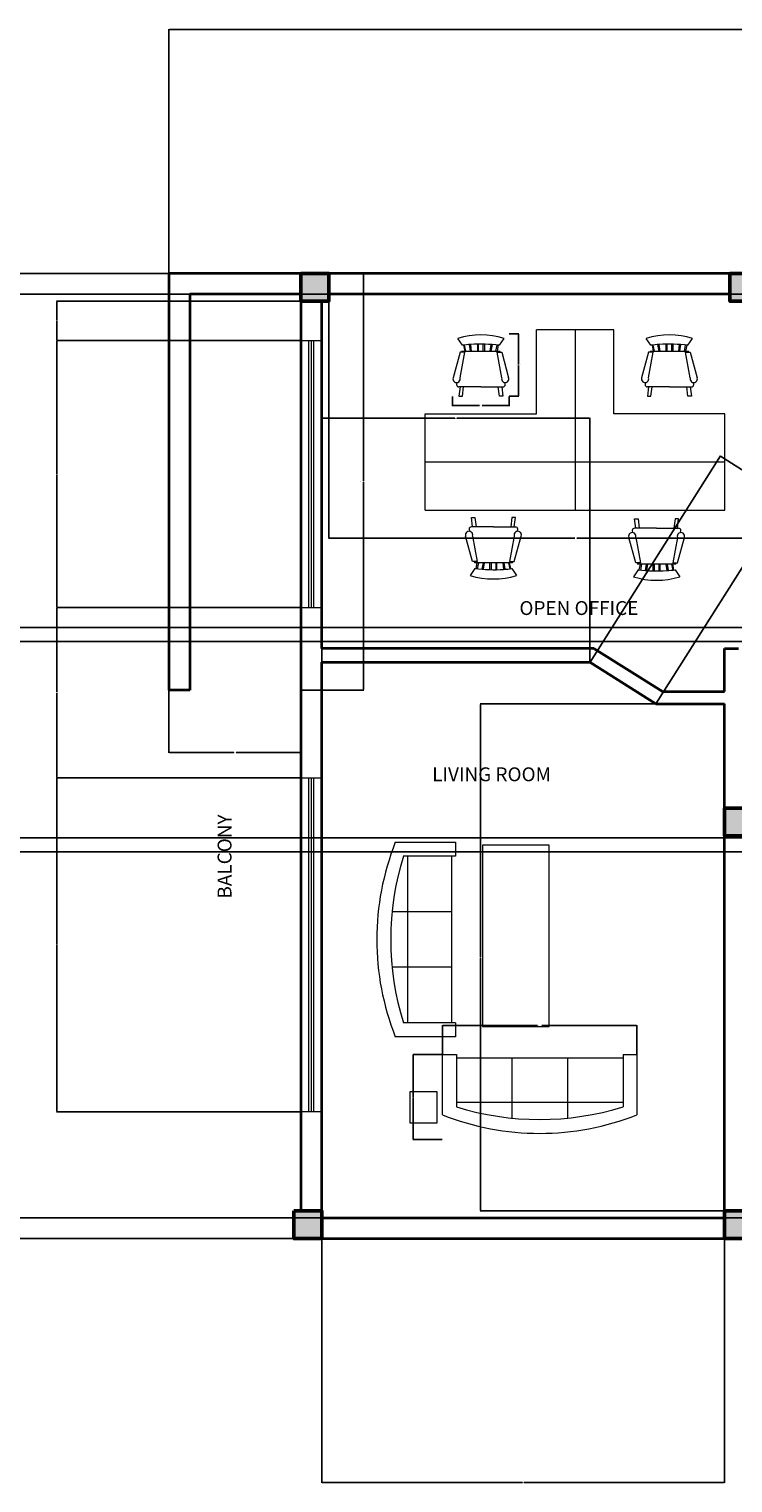
# Model space of a CAD drawing. Units: inches. Extents: x 369 to 4994, y 516 to 1297.
# Tile 4 of 9: x 1148 to 1452, y 516 to 1144. Entities that reach past the tile are written whole.
import ezdxf

# ---------------------------------------------------------------- set-up
doc = ezdxf.new("R2010")
doc.units = ezdxf.units.IN
doc.header["$MEASUREMENT"] = 0
for name, color, linetype, lineweight in [('A-ANNO-DIMS', 2, 'Continuous', 18), ('A-AREA-IDEN', 7, 'Continuous', 18), ('A-COLS', 7, 'Continuous', 50), ('A-FURN', 8, 'Continuous', 18), ('A-GLAZ', 4, 'Continuous', 18), ('A-WALL', 7, 'Continuous', 35)]:
    doc.layers.add(name, color=color, linetype=linetype, lineweight=lineweight)
doc.layers.add('A-COLS-PATT', color=18, linetype='Continuous', lineweight=13, true_color=0x000000)
doc.styles.get("Standard").update_dxf_attribs({"font": 'arial.ttf'})
doc.dimstyles.get("Standard").update_dxf_attribs({"dimtxt": 0.18, "dimasz": 0.18, "dimexe": 0.18, "dimexo": 0.0625, "dimgap": 0.09, "dimtad": 0, "dimtih": 1, "dimtoh": 1, "dimdec": 4, "dimzin": 0, "dimdsep": 46, "dimtxsty": 'Standard', "dimcen": 0.09, "dimadec": 0, "dimazin": 0, "dimtfac": 1, "dimtdec": 4, "dimtofl": 0, "dimtmove": 0, "dimatfit": 3, "dimfxl": 1, "dimtolj": 1, "dimtzin": 0, "dimarcsym": 0})

# ---------------------------------------------------------------- blocks, each defined once
blk = doc.blocks.new('Chair - Rocking')
for p, q in [((-8, -4.5), (-10, -1.5)), ((-7.5, -4.5), (-7, -7)), ((-6.5, -7), (-7.02225, -4.43)), ((-4.5, -7), (-4.96674, -4.19951)), ((-4, -7), (-4.40532, -4.16272)), ((-1.5, -4.05012), (-1.5, -7)), ((-1, -7), (-1, -4.05012)), ((1, -7), (1, -4.04655)), ((1.5, -4.05012), (1.5, -7)), ((4, -7), (4.40187, -4.18694)), ((4.5, -7), (4.96761, -4.19437)), ((6.5, -7), (7, -4.4057)), ((7.5, -4.5), (7, -7)), ((8, -4.5), (10, -1.5)), ((-9, -7.5), (-12, -18.49999)), ((-7, -7.5), (-9, -7.5)), ((-9, -18.49999), (-7, -7.5)), ((-8.23428, -6.99939), (-8.3093, -7.47958)), ((-8.23041, -7), (8.23915, -7)), ((7, -7.5), (9, -7.5)), ((9, -18.49999), (7, -7.5)), ((8.31071, -7.48854), (8.23449, -7.00073)), ((9, -7.5), (12, -18.49999)), ((-10.36644, -20.64523), (-10.5, -21.49999)), ((-9, -22.49999), (-9.5, -26.49999)), ((0, -22.49999), (-9.5, -22.49999)), ((-8, -26.49999), (-7.5, -22.49999)), ((0, -22.49999), (9.5, -22.49999)), ((8, -26.49999), (7.5, -22.49999)), ((9, -22.49999), (9.5, -26.49999)), ((10.5, -21.49999), (10.3575, -20.58798)), ((-9.5, -26.49999), (-8, -26.49999)), ((9.5, -26.49999), (8, -26.49999))]:
    blk.add_line(p, q)
for centre, radius, start, end in [((0, -34.08333), 34.08333, 72.93847, 107.0615), ((0, -68.25004), 64.25, 93.92211, 97.15267), ((0, -68.25004), 64.25, 82.84733, 93.92211), ((-10.5, -18.99999), 1.58114, 161.5651, 18.43495), ((10.5, -18.99999), 1.58114, 161.5651, 18.43495), ((-9.5, -21.49999), 1, 180, 270), ((9.5, -21.49999), 1, 270, 0)]:
    blk.add_arc(centre, radius, start, end)
blk = doc.blocks.new('Sofa - Roundback 7 ft.')
for p, q in [((-36.000027, -34), (-36.000027, -11.4696)), ((-12.00002, -32.4421), (-12.00003, -6.5971)), ((11.99997, -32.4421), (11.99998, -6.5971)), ((35.99998, -34), (35.99998, -11.4696)), ((-35.999844, -13.3819), (35.9998, -13.3819)), ((-36.000027, -32.4421), (35.99998, -32.4421))]:
    blk.add_line(p, q)
for points in [[(-36.000027, -34), (-42.000027, -34), (-42.000027, -8)], [(41.99998, -8), (41.99998, -34), (35.99998, -34)]]:
    blk.add_lwpolyline(points)
for centre, radius, start, end in [((0, -114.25), 114.25, 68.43141, 111.5686), ((-0.00001, -127.1968), 121.1968, 72.72033, 107.2797)]:
    blk.add_arc(centre, radius, start, end)
blk = doc.blocks.new('BALCONY-EDGE')
for p, q in [((57, 180), (0, 180)), ((0, 180), (0, 0)), ((9, 171), (9, 0)), ((57, 171), (9, 171)), ((9, 0), (0, 0))]:
    blk.add_line(p, q)
blk = doc.blocks.new('*D13')
at = {"layer": 'A-ANNO-DIMS', "color": 0, "lineweight": -2, "transparency": 16777216}
for p, q in [((1265.44, 1038.79), (1292.55, 1038.79)), ((1292.37, 1038.61), (1292.37, 948.97)), ((1292.37, 858.97), (1292.37, 948.61)), ((1265.44, 858.79), (1292.55, 858.79))]:
    blk.add_line(p, q, dxfattribs=at)
at = {"layer": 'A-ANNO-DIMS', "color": 0, "transparency": 16777216}
for points in [[(1292.34, 1038.61), (1292.4, 1038.61), (1292.37, 1038.79)], [(1292.34, 858.97), (1292.4, 858.97), (1292.37, 858.79)]]:
    blk.add_solid(points, dxfattribs=at)
at = {"layer": 'Defpoints', "color": 0, "transparency": 16777216}
for p in [(1265.37, 1038.79), (1292.37, 1038.79), (1265.37, 858.79)]:
    blk.add_point(p, dxfattribs=at)
at = {"layer": 'A-ANNO-DIMS', "color": 0, "transparency": 16777216, "insert": (1292.37, 948.79), "char_height": 0.18, "attachment_point": 5}
blk.add_mtext('\\A1;BALCONY EDGE 180 TYP.', dxfattribs=at)
blk = doc.blocks.new('*D14')
at = {"layer": 'A-ANNO-DIMS', "color": 0, "lineweight": -2, "transparency": 16777216}
for p, q in [((1208.37, 858.73), (1208.37, 831.61)), ((1265.37, 858.73), (1265.37, 831.61)), ((1208.55, 831.79), (1236.35, 831.79)), ((1265.19, 831.79), (1237.4, 831.79))]:
    blk.add_line(p, q, dxfattribs=at)
at = {"layer": 'A-ANNO-DIMS', "color": 0, "transparency": 16777216}
for points in [[(1208.55, 831.82), (1208.55, 831.76), (1208.37, 831.79)], [(1265.19, 831.82), (1265.19, 831.76), (1265.37, 831.79)]]:
    blk.add_solid(points, dxfattribs=at)
at = {"layer": 'Defpoints', "color": 0, "transparency": 16777216}
for p in [(1208.37, 858.79), (1265.37, 858.79), (1265.37, 831.79)]:
    blk.add_point(p, dxfattribs=at)
at = {"layer": 'A-ANNO-DIMS', "color": 0, "transparency": 16777216, "insert": (1236.87, 831.79), "char_height": 0.18, "attachment_point": 5}
blk.add_mtext('\\A1;57 TYP.', dxfattribs=at)
blk = doc.blocks.new('*D21')
at = {"layer": 'A-ANNO-DIMS', "color": 0, "lineweight": -2, "transparency": 16777216}
for p, q in [((1326.51, 701.31), (1326.51, 714.03)), ((1326.69, 713.85), (1367.6, 713.85)), ((1410.33, 713.85), (1369.41, 713.85)), ((1410.51, 701.31), (1410.51, 714.03))]:
    blk.add_line(p, q, dxfattribs=at)
at = {"layer": 'A-ANNO-DIMS', "color": 0, "transparency": 16777216}
for points in [[(1326.69, 713.88), (1326.69, 713.82), (1326.51, 713.85)], [(1410.33, 713.88), (1410.33, 713.82), (1410.51, 713.85)]]:
    blk.add_solid(points, dxfattribs=at)
at = {"layer": 'Defpoints', "color": 0, "transparency": 16777216}
for p in [(1326.51, 713.85), (1326.51, 701.25), (1410.51, 701.25)]:
    blk.add_point(p, dxfattribs=at)
at = {"layer": 'A-ANNO-DIMS', "color": 0, "transparency": 16777216, "insert": (1368.51, 713.85), "char_height": 0.18, "attachment_point": 5}
blk.add_mtext('\\A1;SOFA 84 TYP.', dxfattribs=at)
blk = doc.blocks.new('*D22')
at = {"layer": 'A-ANNO-DIMS', "color": 0, "lineweight": -2, "transparency": 16777216}
for p, q in [((1326.44, 701.25), (1313.73, 701.25)), ((1313.91, 701.07), (1313.91, 683.09)), ((1313.91, 664.76), (1313.91, 682.73)), ((1326.44, 664.58), (1313.73, 664.58))]:
    blk.add_line(p, q, dxfattribs=at)
at = {"layer": 'A-ANNO-DIMS', "color": 0, "transparency": 16777216}
for points in [[(1313.88, 701.07), (1313.94, 701.07), (1313.91, 701.25)], [(1313.88, 664.76), (1313.94, 664.76), (1313.91, 664.58)]]:
    blk.add_solid(points, dxfattribs=at)
at = {"layer": 'Defpoints', "color": 0, "transparency": 16777216}
for p in [(1326.51, 701.25), (1313.91, 664.58), (1326.51, 664.58)]:
    blk.add_point(p, dxfattribs=at)
at = {"layer": 'A-ANNO-DIMS', "color": 0, "transparency": 16777216, "insert": (1313.91, 682.91), "char_height": 0.18, "attachment_point": 5}
blk.add_mtext('\\A1;37 TYP.', dxfattribs=at)
blk = doc.blocks.new('*D23')
at = {"layer": 'A-ANNO-DIMS', "color": 0, "lineweight": -2, "transparency": 16777216}
for p, q in [((1355.39, 1012.74), (1359.55, 1012.74)), ((1359.37, 1012.56), (1359.37, 999.42)), ((1359.37, 985.92), (1359.37, 999.06)), ((1355.39, 985.74), (1359.55, 985.74))]:
    blk.add_line(p, q, dxfattribs=at)
at = {"layer": 'A-ANNO-DIMS', "color": 0, "transparency": 16777216}
for points in [[(1359.34, 1012.56), (1359.4, 1012.56), (1359.37, 1012.74)], [(1359.34, 985.92), (1359.4, 985.92), (1359.37, 985.74)]]:
    blk.add_solid(points, dxfattribs=at)
at = {"layer": 'Defpoints', "color": 0, "transparency": 16777216}
for p in [(1355.32, 1012.74), (1359.37, 1012.74), (1355.32, 985.74)]:
    blk.add_point(p, dxfattribs=at)
at = {"layer": 'A-ANNO-DIMS', "color": 0, "transparency": 16777216, "insert": (1359.37, 999.24), "char_height": 0.18, "attachment_point": 5}
blk.add_mtext('\\A1;CHAIR 27 TYP.', dxfattribs=at)
blk = doc.blocks.new('*D24')
at = {"layer": 'A-ANNO-DIMS', "color": 0, "lineweight": -2, "transparency": 16777216}
for p, q in [((1330.89, 985.68), (1330.89, 981.51)), ((1331.07, 981.69), (1342.58, 981.69)), ((1355.14, 981.69), (1343.64, 981.69)), ((1355.32, 985.68), (1355.32, 981.51))]:
    blk.add_line(p, q, dxfattribs=at)
at = {"layer": 'A-ANNO-DIMS', "color": 0, "transparency": 16777216}
for points in [[(1331.07, 981.72), (1331.07, 981.66), (1330.89, 981.69)], [(1355.14, 981.72), (1355.14, 981.66), (1355.32, 981.69)]]:
    blk.add_solid(points, dxfattribs=at)
at = {"layer": 'Defpoints', "color": 0, "transparency": 16777216}
for p in [(1330.89, 985.74), (1355.32, 985.74), (1355.32, 981.69)]:
    blk.add_point(p, dxfattribs=at)
at = {"layer": 'A-ANNO-DIMS', "color": 0, "transparency": 16777216, "insert": (1343.11, 981.69), "char_height": 0.18, "attachment_point": 5}
blk.add_mtext('\\A1;24 TYP.', dxfattribs=at)
blk = doc.blocks.new('*D46')
at = {"layer": 'A-ANNO-DIMS', "color": 0, "lineweight": -2, "transparency": 16777216}
for p, q in [((978.32, 1029.79), (2671.51, 1029.79)), ((2671.33, 1029.61), (2671.33, 957.97)), ((2671.33, 885.97), (2671.33, 957.61)), ((1038.32, 885.79), (2671.51, 885.79))]:
    blk.add_line(p, q, dxfattribs=at)
at = {"layer": 'A-ANNO-DIMS', "color": 0, "transparency": 16777216}
for points in [[(2671.3, 1029.61), (2671.36, 1029.61), (2671.33, 1029.79)], [(2671.3, 885.97), (2671.36, 885.97), (2671.33, 885.79)]]:
    blk.add_solid(points, dxfattribs=at)
at = {"layer": 'Defpoints', "color": 0, "transparency": 16777216}
for p in [(978.26, 1029.79), (2671.33, 1029.79), (1038.26, 885.79)]:
    blk.add_point(p, dxfattribs=at)
at = {"layer": 'A-ANNO-DIMS', "color": 0, "transparency": 16777216, "insert": (2671.33, 957.79), "char_height": 0.18, "attachment_point": 5}
blk.add_mtext('\\A1;144', dxfattribs=at)
blk = doc.blocks.new('*D47')
at = {"layer": 'A-ANNO-DIMS', "color": 0, "lineweight": -2, "transparency": 16777216}
for p, q in [((1038.32, 879.79), (2671.51, 879.79)), ((2671.33, 879.61), (2671.33, 837.52)), ((2671.33, 795.07), (2671.33, 837.16)), ((1035.32, 794.89), (2671.51, 794.89))]:
    blk.add_line(p, q, dxfattribs=at)
at = {"layer": 'A-ANNO-DIMS', "color": 0, "transparency": 16777216}
for points in [[(2671.3, 879.61), (2671.36, 879.61), (2671.33, 879.79)], [(2671.3, 795.07), (2671.36, 795.07), (2671.33, 794.89)]]:
    blk.add_solid(points, dxfattribs=at)
at = {"layer": 'Defpoints', "color": 0, "transparency": 16777216}
for p in [(1038.26, 879.79), (2671.33, 879.79), (1035.26, 794.89)]:
    blk.add_point(p, dxfattribs=at)
at = {"layer": 'A-ANNO-DIMS', "color": 0, "transparency": 16777216, "insert": (2671.33, 837.34), "char_height": 0.18, "attachment_point": 5}
blk.add_mtext('\\A1;84.9', dxfattribs=at)
blk = doc.blocks.new('*D52')
at = {"layer": 'A-ANNO-DIMS', "color": 0, "lineweight": -2, "transparency": 16777216}
for p, q in [((942.32, 788.89), (2671.51, 788.89)), ((2671.33, 788.71), (2671.33, 710.02)), ((2671.33, 630.97), (2671.33, 709.66)), ((1035.32, 630.79), (2671.51, 630.79))]:
    blk.add_line(p, q, dxfattribs=at)
at = {"layer": 'A-ANNO-DIMS', "color": 0, "transparency": 16777216}
for points in [[(2671.3, 788.71), (2671.36, 788.71), (2671.33, 788.89)], [(2671.3, 630.97), (2671.36, 630.97), (2671.33, 630.79)]]:
    blk.add_solid(points, dxfattribs=at)
at = {"layer": 'Defpoints', "color": 0, "transparency": 16777216}
for p in [(942.26, 788.89), (2671.33, 788.89), (1035.26, 630.79)]:
    blk.add_point(p, dxfattribs=at)
at = {"layer": 'A-ANNO-DIMS', "color": 0, "transparency": 16777216, "insert": (2671.33, 709.84), "char_height": 0.18, "attachment_point": 5}
blk.add_mtext('\\A1;158.1', dxfattribs=at)
blk = doc.blocks.new('*D74')
at = {"layer": 'A-ANNO-DIMS', "color": 0, "lineweight": -2, "transparency": 16777216}
for p, q in [((1208.37, 1038.85), (1208.37, 1144.37)), ((1208.55, 1144.19), (1494.58, 1144.19)), ((1781.19, 1144.19), (1495.16, 1144.19)), ((1781.37, 1038.85), (1781.37, 1144.37))]:
    blk.add_line(p, q, dxfattribs=at)
at = {"layer": 'A-ANNO-DIMS', "color": 0, "transparency": 16777216}
for points in [[(1208.55, 1144.22), (1208.55, 1144.16), (1208.37, 1144.19)], [(1781.19, 1144.22), (1781.19, 1144.16), (1781.37, 1144.19)]]:
    blk.add_solid(points, dxfattribs=at)
at = {"layer": 'Defpoints', "color": 0, "transparency": 16777216}
for p in [(1781.37, 1144.19), (1208.37, 1038.79), (1781.37, 1038.79)]:
    blk.add_point(p, dxfattribs=at)
at = {"layer": 'A-ANNO-DIMS', "color": 0, "transparency": 16777216, "insert": (1494.87, 1144.19), "char_height": 0.18, "attachment_point": 5}
blk.add_mtext('\\A1;573', dxfattribs=at)
blk = doc.blocks.new('*D75')
at = {"layer": 'A-ANNO-DIMS', "color": 0, "lineweight": -2, "transparency": 16777216}
for p, q in [((1208.31, 1038.79), (368.68, 1038.79)), ((368.86, 1038.61), (368.86, 830.47)), ((368.86, 621.97), (368.86, 830.11)), ((1262.31, 621.79), (368.68, 621.79))]:
    blk.add_line(p, q, dxfattribs=at)
at = {"layer": 'A-ANNO-DIMS', "color": 0, "transparency": 16777216}
for points in [[(368.83, 1038.61), (368.89, 1038.61), (368.86, 1038.79)], [(368.83, 621.97), (368.89, 621.97), (368.86, 621.79)]]:
    blk.add_solid(points, dxfattribs=at)
at = {"layer": 'Defpoints', "color": 0, "transparency": 16777216}
for p in [(368.86, 1038.79), (1208.37, 1038.79), (1262.37, 621.79)]:
    blk.add_point(p, dxfattribs=at)
at = {"layer": 'A-ANNO-DIMS', "color": 0, "transparency": 16777216, "insert": (368.86, 830.29), "char_height": 0.18, "attachment_point": 5}
blk.add_mtext('\\A1;417', dxfattribs=at)
blk = doc.blocks.new('*D76')
at = {"layer": 'A-ANNO-DIMS', "color": 0, "lineweight": -2, "transparency": 16777216}
for p, q in [((1277.37, 1029.73), (1277.37, 924.21)), ((1490.89, 1029.73), (1490.89, 924.21)), ((1277.55, 924.39), (1383.74, 924.39)), ((1490.71, 924.39), (1384.53, 924.39))]:
    blk.add_line(p, q, dxfattribs=at)
at = {"layer": 'A-ANNO-DIMS', "color": 0, "transparency": 16777216}
for points in [[(1277.55, 924.42), (1277.55, 924.36), (1277.37, 924.39)], [(1490.71, 924.42), (1490.71, 924.36), (1490.89, 924.39)]]:
    blk.add_solid(points, dxfattribs=at)
at = {"layer": 'Defpoints', "color": 0, "transparency": 16777216}
for p in [(1277.37, 1029.79), (1490.89, 1029.79), (1277.37, 924.39)]:
    blk.add_point(p, dxfattribs=at)
at = {"layer": 'A-ANNO-DIMS', "color": 0, "transparency": 16777216, "insert": (1384.13, 924.39), "char_height": 0.18, "attachment_point": 5}
blk.add_mtext('\\A1;213.5', dxfattribs=at)
blk = doc.blocks.new('*D81')
at = {"layer": 'A-ANNO-DIMS', "color": 0, "lineweight": -2, "transparency": 16777216}
for p, q in [((1274.37, 630.73), (1274.37, 516.21)), ((1448.37, 630.73), (1448.37, 516.21)), ((1274.55, 516.39), (1361.09, 516.39)), ((1448.19, 516.39), (1361.65, 516.39))]:
    blk.add_line(p, q, dxfattribs=at)
at = {"layer": 'A-ANNO-DIMS', "color": 0, "transparency": 16777216}
for points in [[(1274.55, 516.42), (1274.55, 516.36), (1274.37, 516.39)], [(1448.19, 516.42), (1448.19, 516.36), (1448.37, 516.39)]]:
    blk.add_solid(points, dxfattribs=at)
at = {"layer": 'Defpoints', "color": 0, "transparency": 16777216}
for p in [(1274.37, 630.79), (1448.37, 630.79), (1448.37, 516.39)]:
    blk.add_point(p, dxfattribs=at)
at = {"layer": 'A-ANNO-DIMS', "color": 0, "transparency": 16777216, "insert": (1361.37, 516.39), "char_height": 0.18, "attachment_point": 5}
blk.add_mtext('\\A1;174', dxfattribs=at)
blk = doc.blocks.new('*D87')
at = {"layer": 'A-ANNO-DIMS', "color": 0, "lineweight": -2, "transparency": 16777216}
for p, q in [((1274.37, 870.85), (1274.37, 976.37)), ((1274.55, 976.19), (1331.85, 976.19)), ((1390.05, 976.19), (1332.76, 976.19)), ((1390.23, 870.85), (1390.23, 976.37))]:
    blk.add_line(p, q, dxfattribs=at)
at = {"layer": 'A-ANNO-DIMS', "color": 0, "transparency": 16777216}
for points in [[(1274.55, 976.22), (1274.55, 976.16), (1274.37, 976.19)], [(1390.05, 976.22), (1390.05, 976.16), (1390.23, 976.19)]]:
    blk.add_solid(points, dxfattribs=at)
at = {"layer": 'Defpoints', "color": 0, "transparency": 16777216}
for p in [(1390.23, 976.19), (1274.37, 870.79), (1390.23, 870.79)]:
    blk.add_point(p, dxfattribs=at)
at = {"layer": 'A-ANNO-DIMS', "color": 0, "transparency": 16777216, "insert": (1332.3, 976.19), "char_height": 0.18, "attachment_point": 5}
blk.add_mtext('\\A1;115.86', dxfattribs=at)
blk = doc.blocks.new('*D88')
at = {"layer": 'A-ANNO-DIMS', "color": 0, "lineweight": -2, "transparency": 16777216}
for p, q in [((1390.27, 870.84), (1446.63, 960.04)), ((1446.68, 959.8), (1460.49, 951.07)), ((1474.87, 941.99), (1461.06, 950.71)), ((1418.75, 852.84), (1475.12, 942.04))]:
    blk.add_line(p, q, dxfattribs=at)
at = {"layer": 'A-ANNO-DIMS', "color": 0, "transparency": 16777216}
for points in [[(1446.7, 959.82), (1446.67, 959.77), (1446.53, 959.89)], [(1474.88, 942.01), (1474.85, 941.96), (1475.02, 941.89)]]:
    blk.add_solid(points, dxfattribs=at)
at = {"layer": 'Defpoints', "color": 0, "transparency": 16777216}
for p in [(1475.02, 941.89), (1390.23, 870.79), (1418.72, 852.79)]:
    blk.add_point(p, dxfattribs=at)
at = {"layer": 'A-ANNO-DIMS', "color": 0, "transparency": 16777216, "insert": (1460.78, 950.89), "char_height": 0.18, "attachment_point": 5}
blk.add_mtext('\\A1;33.7', dxfattribs=at)
blk = doc.blocks.new('*D89')
at = {"layer": 'A-ANNO-DIMS', "color": 0, "lineweight": -2, "transparency": 16777216}
for p, q in [((1448.31, 852.79), (1342.79, 852.79)), ((1342.97, 852.61), (1342.97, 743.47)), ((1342.97, 633.97), (1342.97, 743.11)), ((1448.31, 633.79), (1342.79, 633.79))]:
    blk.add_line(p, q, dxfattribs=at)
at = {"layer": 'A-ANNO-DIMS', "color": 0, "transparency": 16777216}
for points in [[(1342.94, 852.61), (1343, 852.61), (1342.97, 852.79)], [(1342.94, 633.97), (1343, 633.97), (1342.97, 633.79)]]:
    blk.add_solid(points, dxfattribs=at)
at = {"layer": 'Defpoints', "color": 0, "transparency": 16777216}
for p in [(1342.97, 852.79), (1448.37, 852.79), (1448.37, 633.79)]:
    blk.add_point(p, dxfattribs=at)
at = {"layer": 'A-ANNO-DIMS', "color": 0, "transparency": 16777216, "insert": (1342.97, 743.29), "char_height": 0.18, "attachment_point": 5}
blk.add_mtext('\\A1;219', dxfattribs=at)
blk = doc.blocks.new('*D90')
at = {"layer": 'A-ANNO-DIMS', "color": 0, "lineweight": -2, "transparency": 16777216}
for p, q in [((1265.31, 1026.79), (1159.79, 1026.79)), ((1159.97, 1026.61), (1159.97, 1018.46)), ((1159.97, 1009.95), (1159.97, 1018.1)), ((1265.31, 1009.77), (1159.79, 1009.77))]:
    blk.add_line(p, q, dxfattribs=at)
at = {"layer": 'A-ANNO-DIMS', "color": 0, "transparency": 16777216}
for points in [[(1159.94, 1026.61), (1160, 1026.61), (1159.97, 1026.79)], [(1159.94, 1009.95), (1160, 1009.95), (1159.97, 1009.77)]]:
    blk.add_solid(points, dxfattribs=at)
at = {"layer": 'Defpoints', "color": 0, "transparency": 16777216}
for p in [(1159.97, 1026.79), (1265.37, 1026.79), (1265.37, 1009.77)]:
    blk.add_point(p, dxfattribs=at)
at = {"layer": 'A-ANNO-DIMS', "color": 0, "transparency": 16777216, "insert": (1159.97, 1018.28), "char_height": 0.18, "attachment_point": 5}
blk.add_mtext('\\A1;17.023', dxfattribs=at)
blk = doc.blocks.new('*D91')
at = {"layer": 'A-ANNO-DIMS', "color": 0, "lineweight": -2, "transparency": 16777216}
for p, q in [((1265.31, 1009.77), (1159.79, 1009.77)), ((1159.97, 1009.59), (1159.97, 952.25)), ((1159.97, 894.56), (1159.97, 951.89)), ((1265.31, 894.38), (1159.79, 894.38))]:
    blk.add_line(p, q, dxfattribs=at)
at = {"layer": 'A-ANNO-DIMS', "color": 0, "transparency": 16777216}
for points in [[(1159.94, 1009.59), (1160, 1009.59), (1159.97, 1009.77)], [(1159.94, 894.56), (1160, 894.56), (1159.97, 894.38)]]:
    blk.add_solid(points, dxfattribs=at)
at = {"layer": 'Defpoints', "color": 0, "transparency": 16777216}
for p in [(1159.97, 1009.77), (1265.37, 1009.77), (1265.37, 894.38)]:
    blk.add_point(p, dxfattribs=at)
at = {"layer": 'A-ANNO-DIMS', "color": 0, "transparency": 16777216, "insert": (1159.97, 952.07), "char_height": 0.18, "attachment_point": 5}
blk.add_mtext('\\A1;115.39', dxfattribs=at)
blk = doc.blocks.new('*D92')
at = {"layer": 'A-ANNO-DIMS', "color": 0, "lineweight": -2, "transparency": 16777216}
for p, q in [((1265.31, 894.38), (1159.79, 894.38)), ((1159.97, 894.2), (1159.97, 857.81)), ((1159.97, 821.05), (1159.97, 857.44)), ((1265.31, 820.87), (1159.79, 820.87))]:
    blk.add_line(p, q, dxfattribs=at)
at = {"layer": 'A-ANNO-DIMS', "color": 0, "transparency": 16777216}
for points in [[(1159.94, 894.2), (1160, 894.2), (1159.97, 894.38)], [(1159.94, 821.05), (1160, 821.05), (1159.97, 820.87)]]:
    blk.add_solid(points, dxfattribs=at)
at = {"layer": 'Defpoints', "color": 0, "transparency": 16777216}
for p in [(1159.97, 894.38), (1265.37, 894.38), (1265.37, 820.87)]:
    blk.add_point(p, dxfattribs=at)
at = {"layer": 'A-ANNO-DIMS', "color": 0, "transparency": 16777216, "insert": (1159.97, 857.62), "char_height": 0.18, "attachment_point": 5}
blk.add_mtext('\\A1;73.51', dxfattribs=at)
blk = doc.blocks.new('*D93')
at = {"layer": 'A-ANNO-DIMS', "color": 0, "lineweight": -2, "transparency": 16777216}
for p, q in [((1265.31, 820.87), (1159.79, 820.87)), ((1159.97, 820.69), (1159.97, 748.88)), ((1159.97, 676.7), (1159.97, 748.51)), ((1265.31, 676.52), (1159.79, 676.52))]:
    blk.add_line(p, q, dxfattribs=at)
at = {"layer": 'A-ANNO-DIMS', "color": 0, "transparency": 16777216}
for points in [[(1159.94, 820.69), (1160, 820.69), (1159.97, 820.87)], [(1159.94, 676.7), (1160, 676.7), (1159.97, 676.52)]]:
    blk.add_solid(points, dxfattribs=at)
at = {"layer": 'Defpoints', "color": 0, "transparency": 16777216}
for p in [(1159.97, 820.87), (1265.37, 820.87), (1265.37, 676.52)]:
    blk.add_point(p, dxfattribs=at)
at = {"layer": 'A-ANNO-DIMS', "color": 0, "transparency": 16777216, "insert": (1159.97, 748.69), "char_height": 0.18, "attachment_point": 5}
blk.add_mtext('\\A1;144.35', dxfattribs=at)
blk = doc.blocks.new('*D98')
at = {"layer": 'A-ANNO-DIMS', "color": 0, "lineweight": -2, "transparency": 16777216}
for p, q in [((1992.86, 1038.79), (368.68, 1038.79)), ((368.86, 1038.61), (368.86, 830.47)), ((368.86, 621.97), (368.86, 830.11)), ((2046.86, 621.79), (368.68, 621.79))]:
    blk.add_line(p, q, dxfattribs=at)
at = {"layer": 'A-ANNO-DIMS', "color": 0, "transparency": 16777216}
for points in [[(368.83, 1038.61), (368.89, 1038.61), (368.86, 1038.79)], [(368.83, 621.97), (368.89, 621.97), (368.86, 621.79)]]:
    blk.add_solid(points, dxfattribs=at)
at = {"layer": 'Defpoints', "color": 0, "transparency": 16777216}
for p in [(368.86, 1038.79), (1992.93, 1038.79), (2046.93, 621.79)]:
    blk.add_point(p, dxfattribs=at)
at = {"layer": 'A-ANNO-DIMS', "color": 0, "transparency": 16777216, "insert": (368.86, 830.29), "char_height": 0.18, "attachment_point": 5}
blk.add_mtext('\\A1;417', dxfattribs=at)

msp = doc.modelspace()

# ---------------------------------------------------------------- hatches: boundary and pattern name
at = {"layer": 'A-COLS-PATT'}
h = msp.add_hatch(color=256, dxfattribs=at)
h.dxf.hatch_style = 1
h.paths.add_polyline_path([(540.2581, 633.7894), (528.2581, 633.7894), (528.2581, 621.7894), (540.2581, 621.7894)])
h.paths.add_polyline_path([(726.2581, 633.7894), (714.2581, 633.7894), (714.2581, 621.7894), (726.2581, 621.7894)])
h.paths.add_polyline_path([(918.2581, 633.7894), (906.2581, 633.7894), (906.2581, 621.7894), (918.2581, 621.7894)])
h.paths.add_polyline_path([(1047.2581, 633.7894), (1035.2581, 633.7894), (1035.2581, 621.7894), (1047.2581, 621.7894)])
h.paths.add_polyline_path([(1047.2581, 798.6977), (1035.2581, 798.6977), (1035.2581, 786.6977), (1047.2581, 786.6977)])
h.paths.add_polyline_path([(918.2581, 795.7894), (906.2581, 795.7894), (906.2581, 783.7894), (918.2581, 783.7894)])
h.paths.add_polyline_path([(726.2581, 795.7894), (714.2581, 795.7894), (714.2581, 783.7894), (726.2581, 783.7894)])
h.paths.add_polyline_path([(1047.2581, 1038.7894), (1035.2581, 1038.7894), (1035.2581, 1026.7894), (1047.2581, 1026.7894)])
h.paths.add_polyline_path([(855.044, 1038.7894), (843.044, 1038.7894), (843.044, 1026.7894), (855.044, 1026.7894)])
h.paths.add_polyline_path([(728.5536, 1038.7894), (716.5536, 1038.7894), (716.5536, 1026.7894), (728.5536, 1026.7894)])
h.paths.add_polyline_path([(543.2581, 1038.7894), (531.2581, 1038.7894), (531.2581, 1026.7894), (543.2581, 1026.7894)])
h.paths.add_polyline_path([(543.2581, 792.9013), (531.2581, 792.9013), (531.2581, 780.9013), (543.2581, 780.9013), (543.2581, 783.7894)])
h.paths.add_polyline_path([(1274.3738, 633.7894), (1262.3738, 633.7894), (1262.3738, 621.7894), (1274.3738, 621.7894)])
h.paths.add_polyline_path([(1460.3738, 633.7894), (1448.3738, 633.7894), (1448.3738, 621.7894), (1460.3738, 621.7894)])
h.paths.add_polyline_path([(1652.3738, 633.7894), (1640.3738, 633.7894), (1640.3738, 621.7894), (1652.3738, 621.7894)])
h.paths.add_polyline_path([(1781.3738, 633.7894), (1769.3738, 633.7894), (1769.3738, 621.7894), (1781.3738, 621.7894)])
h.paths.add_polyline_path([(1781.3738, 1038.7894), (1769.3738, 1038.7894), (1769.3738, 1026.7894), (1781.3738, 1026.7894)])
h.paths.add_polyline_path([(1625.484, 1038.7894), (1613.484, 1038.7894), (1613.484, 1026.7894), (1615.6962, 1026.7894), (1625.484, 1026.7894)])
h.paths.add_polyline_path([(1462.6692, 1038.7894), (1450.6692, 1038.7894), (1450.6692, 1026.7894), (1462.6692, 1026.7894)])
h.paths.add_polyline_path([(1277.3738, 1038.7894), (1265.3738, 1038.7894), (1265.3738, 1026.7894), (1277.3738, 1026.7894)])
h.paths.add_polyline_path([(1460.3738, 807.7894), (1448.3738, 807.7894), (1448.3738, 795.7894), (1460.3738, 795.7894)])
h.paths.add_polyline_path([(1652.3738, 807.7894), (1640.3738, 807.7894), (1640.3738, 795.7894), (1652.3738, 795.7894)])
h.paths.add_polyline_path([(2244.9265, 633.7894), (2232.9265, 633.7894), (2232.9265, 621.7894), (2244.9265, 621.7894)])
h.paths.add_polyline_path([(2058.9265, 633.7894), (2046.9265, 633.7894), (2046.9265, 621.7894), (2058.9265, 621.7894)])
h.paths.add_polyline_path([(2436.9265, 633.7894), (2424.9265, 633.7894), (2424.9265, 621.7894), (2436.9265, 621.7894)])
h.paths.add_polyline_path([(2565.9265, 633.7894), (2553.9265, 633.7894), (2553.9265, 621.7894), (2565.9265, 621.7894)])
h.paths.add_polyline_path([(2565.9265, 798.6977), (2553.9265, 798.6977), (2553.9265, 786.6977), (2565.9265, 786.6977)])
h.paths.add_polyline_path([(2565.9265, 1038.7894), (2553.9265, 1038.7894), (2553.9265, 1026.7894), (2565.9265, 1026.7894)])
h.paths.add_polyline_path([(2436.9265, 1038.7894), (2424.9265, 1038.7894), (2424.9265, 1026.7894), (2436.9265, 1026.7894)])
h.paths.add_polyline_path([(2247.222, 1038.7894), (2235.222, 1038.7894), (2235.222, 1026.7894), (2247.222, 1026.7894)])
h.paths.add_polyline_path([(2061.9265, 1038.7894), (2049.9265, 1038.7894), (2049.9265, 1026.7894), (2061.9265, 1026.7894)])

# ---------------------------------------------------------------- linework, layer by layer
at = {"layer": 'A-COLS'}
for points in [[(1265.3738, 1038.7894), (1277.3738, 1038.7894), (1277.3738, 1026.7894), (1265.3738, 1026.7894)], [(1450.6692, 1038.7894), (1462.6692, 1038.7894), (1462.6692, 1026.7894), (1450.6692, 1026.7894)], [(1448.3738, 807.7894), (1460.3738, 807.7894), (1460.3738, 795.7894), (1448.3738, 795.7894)], [(1262.3738, 633.7894), (1274.3738, 633.7894), (1274.3738, 621.7894), (1262.3738, 621.7894)], [(1448.3738, 633.7894), (1460.3738, 633.7894), (1460.3738, 621.7894), (1448.3738, 621.7894)]]:
    msp.add_lwpolyline(points, close=True, dxfattribs=at)
at = {"layer": 'A-FURN'}
for p, q in [((1367.1047, 978.1573), (1367.1047, 1014.4875)), ((1400.5573, 1014.4875), (1367.1047, 1014.4875)), ((1383.831, 1014.4875), (1383.831, 936.4987)), ((1400.5573, 978.1573), (1400.5573, 1014.4875)), ((1319.1076, 936.4987), (1319.1076, 978.1573)), ((1319.1076, 978.1573), (1367.1047, 978.1573)), ((1448.5544, 978.1573), (1400.5573, 978.1573)), ((1448.5544, 936.4987), (1448.5544, 978.1573)), ((1319.1076, 957.328), (1448.5544, 957.328)), ((1319.1076, 936.4987), (1448.5544, 936.4987))]:
    msp.add_line(p, q, dxfattribs=at)
for points in [[(1343.7905, 713.4743), (1372.6633, 713.4743), (1372.6633, 791.7062), (1343.7905, 791.7062)], [(1312.4848, 671.8573), (1324.2157, 671.8573), (1324.2157, 685.1152), (1312.4848, 685.1152)]]:
    msp.add_lwpolyline(points, close=True, dxfattribs=at)
at = {"layer": 'A-GLAZ'}
for p, q in [((1268.7977, 894.3793), (1268.7977, 1009.766)), ((1269.8738, 894.3793), (1269.8738, 1009.766)), ((1270.9499, 894.3793), (1270.9499, 1009.766)), ((1268.7977, 676.5162), (1268.7977, 820.8704)), ((1269.8738, 676.5162), (1269.8738, 820.8704)), ((1270.9499, 676.5162), (1270.9499, 820.8704))]:
    msp.add_line(p, q, dxfattribs=at)
for points in [[(1265.3738, 1009.766), (1274.3738, 1009.766), (1274.3738, 894.3793), (1265.3738, 894.3793)], [(1274.3738, 676.5162), (1265.3738, 676.5162), (1265.3738, 820.8704), (1274.3738, 820.8704)]]:
    msp.add_lwpolyline(points, close=True, dxfattribs=at)
at = {"layer": 'A-WALL'}
for p, q in [((1772.3738, 1038.7894), (1265.3738, 1038.7894)), ((1265.3738, 1029.7894), (1265.3738, 633.7894)), ((1274.3738, 876.7894), (1274.3738, 1026.7894)), ((1450.6692, 1029.7894), (1277.3738, 1029.7894)), ((1391.9688, 876.7894), (1274.3738, 876.7894)), ((1391.9688, 876.7894), (1421.5035, 858.1277)), ((1448.3738, 876.7894), (1454.3738, 876.7894)), ((1448.3738, 870.7894), (1448.3738, 876.7894)), ((1274.3738, 633.7894), (1274.3738, 870.7894)), ((1274.3738, 870.7894), (1390.232, 870.7894)), ((1390.232, 870.7894), (1418.7195, 852.7894)), ((1448.3738, 858.1277), (1448.3738, 870.7894)), ((1421.5035, 858.1277), (1448.3738, 858.1277)), ((1418.7195, 852.7894), (1448.3738, 852.7894)), ((1448.3738, 630.7894), (1448.3738, 852.7894)), ((1274.3738, 630.7894), (1394.3738, 630.7894)), ((1394.3738, 630.7894), (1448.3738, 630.7894)), ((1274.3738, 621.7894), (1394.3738, 621.7894)), ((1394.3738, 621.7894), (1448.3738, 621.7894))]:
    msp.add_line(p, q, dxfattribs=at)

# ---------------------------------------------------------------- block references
at = {"layer": 'A-FURN'}
for p in [(1343.1062, 1012.2406), (1424.5558, 1012.2406)]:
    msp.add_blockref('Chair - Rocking', p, dxfattribs=at)
for name, p, rotation in [('Chair - Rocking', (1348.5241, 906.7805), 180), ('Chair - Rocking', (1419.0201, 906.2215), 180), ('Sofa - Roundback 7 ft.', (1298.136, 750.9881), 90), ('Sofa - Roundback 7 ft.', (1368.5058, 667.246), 180)]:
    msp.add_blockref(name, p, dxfattribs=dict(at, rotation=rotation))
at = {"layer": 'A-WALL'}
msp.add_blockref('BALCONY-EDGE', (1208.3737, 858.789), dxfattribs=at)

# ---------------------------------------------------------------- texts
at = {"layer": 'A-AREA-IDEN'}
for s, p in [('OPEN OFFICE', (1359.7527, 891.218)), ('LIVING ROOM ', (1322.0716, 819.3777))]:
    msp.add_text(s, height=6, dxfattribs=at).set_placement(p)
msp.add_text('BALCONY ', height=6, rotation=90, dxfattribs=at).set_placement((1235.3859, 768.6802))

# ---------------------------------------------------------------- dimensions: what is measured, and where the dimension line sits
at = {"layer": 'A-ANNO-DIMS'}
for base, p1, p2, override, picture, middle in [((1781.3738, 1144.1894), (1208.3738, 1038.7894), (1781.3738, 1038.7894), {"dimdec": 0, "dimlfac": 1, "dimrnd": 0, "dimzin": 0, "dimdsep": 46, "dimlunit": 2}, '*D74', (1494.8738, 1144.1894)), ((1390.232, 976.1894), (1274.3738, 870.7894), (1390.232, 870.7894), {"dimdec": 2, "dimlfac": 1, "dimrnd": 0, "dimzin": 0, "dimdsep": 46, "dimlunit": 2}, '*D87', (1332.3029, 976.1894)), ((1448.3738, 516.3894), (1274.3738, 630.7894), (1448.3738, 630.7894), {"dimdec": 0, "dimlfac": 1, "dimrnd": 0, "dimzin": 0, "dimdsep": 46, "dimlunit": 2}, '*D81', (1361.3738, 516.3894))]:
    dim = msp.add_linear_dim(base=base, p1=p1, p2=p2, dimstyle='Standard', override=override, dxfattribs=at)
    dim.commit()
    dim.dimension.update_dxf_attribs({"geometry": picture, "text_midpoint": middle})
for base, p1, p2, angle, override, picture, middle in [((368.8581, 1038.7894), (1262.3738, 621.7894), (1208.3738, 1038.7894), 90, {"dimdec": 0, "dimlfac": 1, "dimrnd": 0, "dimzin": 0, "dimdsep": 46, "dimlunit": 2}, '*D75', (368.8581, 830.2894)), ((368.8581, 1038.7894), (2046.9265, 621.7894), (1992.9265, 1038.7894), 90, {"dimdec": 0, "dimlfac": 1, "dimrnd": 0, "dimzin": 0, "dimdsep": 46, "dimlunit": 2}, '*D98', (368.8581, 830.2894)), ((2671.3265, 1029.7894), (1038.2581, 885.7894), (978.2581, 1029.7894), 90, {"dimdec": 0, "dimlfac": 1, "dimrnd": 0, "dimzin": 0, "dimdsep": 46, "dimlunit": 2}, '*D46', (2671.3265, 957.7894)), ((1159.9738, 1026.7894), (1265.3738, 1009.766), (1265.3738, 1026.7894), 90, {"dimdec": 3, "dimlfac": 1, "dimrnd": 0, "dimzin": 0, "dimdsep": 46, "dimlunit": 2}, '*D90', (1159.9738, 1018.2777)), ((1277.3738, 924.3894), (1490.89, 1029.7894), (1277.3738, 1029.7894), 180, {"dimdec": 1, "dimlfac": 1, "dimrnd": 0, "dimzin": 0, "dimdsep": 46, "dimlunit": 2}, '*D76', (1384.1319, 924.3894)), ((1159.9738, 1009.766), (1265.3738, 894.3793), (1265.3738, 1009.766), 90, {"dimdec": 2, "dimlfac": 1, "dimrnd": 0, "dimzin": 0, "dimdsep": 46, "dimlunit": 2}, '*D91', (1159.9738, 952.0727)), ((1475.0201, 941.8927), (1390.232, 870.7894), (1418.7195, 852.7894), 327.7129888, {"dimdec": 1, "dimlfac": 1, "dimrnd": 0, "dimzin": 0, "dimdsep": 46, "dimlunit": 2}, '*D88', (1460.7763, 950.8927)), ((1159.9738, 894.3793), (1265.3738, 820.8704), (1265.3738, 894.3793), 90, {"dimdec": 2, "dimlfac": 1, "dimrnd": 0, "dimzin": 0, "dimdsep": 46, "dimlunit": 2}, '*D92', (1159.9738, 857.6249)), ((2671.3265, 879.7894), (1035.2581, 794.8925), (1038.2581, 879.7894), 90, {"dimdec": 1, "dimlfac": 1, "dimrnd": 0, "dimzin": 0, "dimdsep": 46, "dimlunit": 2}, '*D47', (2671.3265, 837.3409)), ((1342.9738, 852.7894), (1448.3738, 633.7894), (1448.3738, 852.7894), 90, {"dimdec": 0, "dimlfac": 1, "dimrnd": 0, "dimzin": 0, "dimdsep": 46, "dimlunit": 2}, '*D89', (1342.9738, 743.2894)), ((1159.9738, 820.8704), (1265.3738, 676.5162), (1265.3738, 820.8704), 90, {"dimdec": 2, "dimlfac": 1, "dimrnd": 0, "dimzin": 0, "dimdsep": 46, "dimlunit": 2}, '*D93', (1159.9738, 748.6933)), ((2671.3265, 788.8925), (1035.2581, 630.7894), (942.2581, 788.8925), 90, {"dimdec": 1, "dimlfac": 1, "dimrnd": 0, "dimzin": 0, "dimdsep": 46, "dimlunit": 2}, '*D52', (2671.3265, 709.8409))]:
    dim = msp.add_linear_dim(base=base, p1=p1, p2=p2, angle=angle, dimstyle='Standard', override=override, dxfattribs=at)
    dim.commit()
    dim.dimension.update_dxf_attribs({"geometry": picture, "text_midpoint": middle})
for base, p1, p2, angle, text, picture, middle in [((1292.3738, 1038.7894), (1265.3738, 858.7894), (1265.3738, 1038.7894), 90, 'BALCONY EDGE <> TYP.', '*D13', (1292.3738, 948.7894)), ((1359.3737, 1012.7406), (1355.3237, 985.7406), (1355.3237, 1012.7406), 90, 'CHAIR <> TYP.', '*D23', (1359.3737, 999.2406)), ((1326.5058, 713.846), (1410.5058, 701.246), (1326.5058, 701.246), 180, 'SOFA <> TYP.', '*D21', (1368.5058, 713.846)), ((1313.9058, 664.5793), (1326.5058, 701.246), (1326.5058, 664.5793), 270, '<> TYP.', '*D22', (1313.9058, 682.9127))]:
    dim = msp.add_linear_dim(base=base, p1=p1, p2=p2, angle=angle, text=text, dimstyle='Standard', override={"dimdec": 0, "dimlfac": 1, "dimrnd": 0, "dimzin": 0, "dimdsep": 46, "dimlunit": 2}, dxfattribs=at)
    dim.commit()
    dim.dimension.update_dxf_attribs({"geometry": picture, "text_midpoint": middle})
for base, p1, p2, picture, middle in [((1355.3237, 981.6906), (1330.8886, 985.7406), (1355.3237, 985.7406), '*D24', (1343.1062, 981.6906)), ((1265.3738, 831.7894), (1208.3738, 858.7894), (1265.3738, 858.7894), '*D14', (1236.8738, 831.7894))]:
    dim = msp.add_linear_dim(base=base, p1=p1, p2=p2, text='<> TYP.', dimstyle='Standard', override={"dimdec": 0, "dimlfac": 1, "dimrnd": 0, "dimzin": 0, "dimdsep": 46, "dimlunit": 2}, dxfattribs=at)
    dim.commit()
    dim.dimension.update_dxf_attribs({"geometry": picture, "text_midpoint": middle})

doc.saveas('drawing.dxf')
